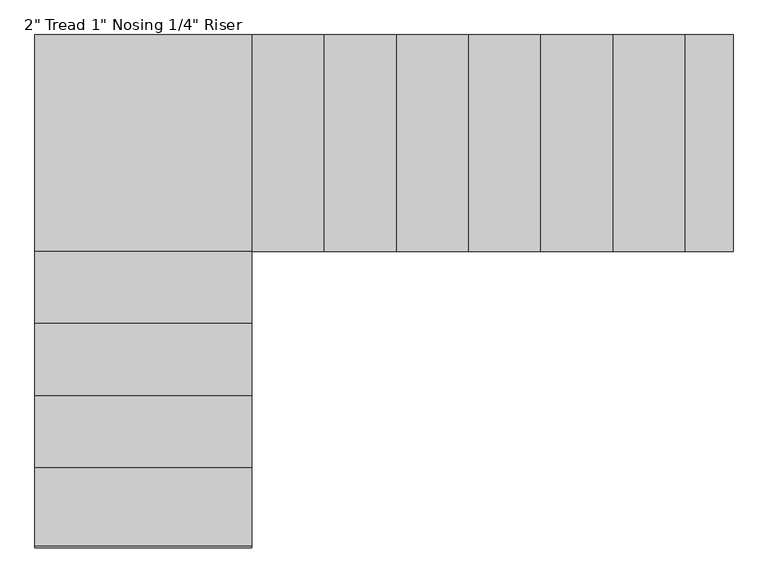
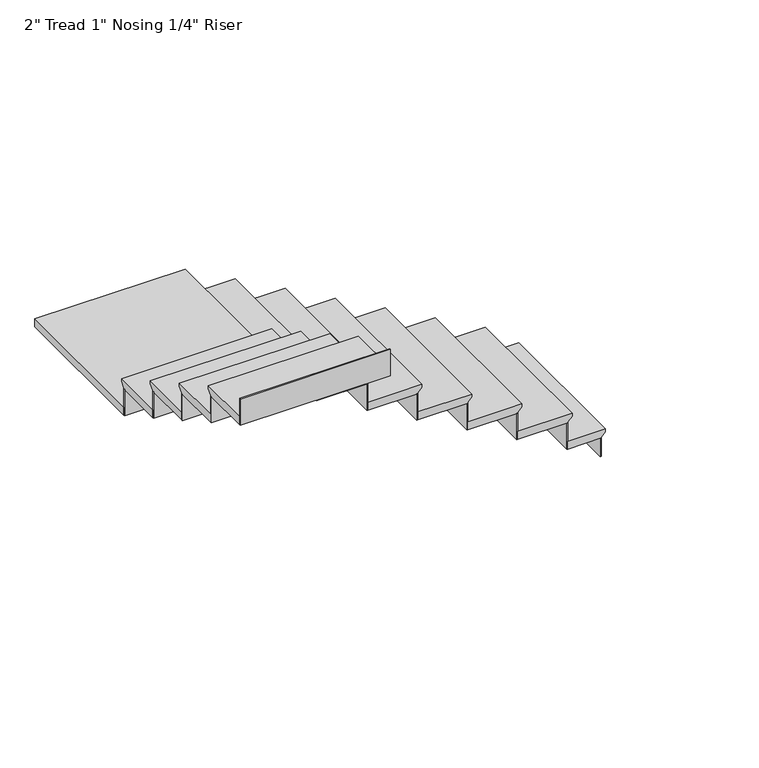
"""IFC4 building model written with IfcOpenShell, lengths in millimetres: stair flight geometry."""

from ifc_helpers import new_model, si_unit, origin, place, context, project, spatial, faceted_brep, source, transform, mapped, element, save


def stair_flight_1226b75b(model_context):
    return source(origin(), model_context, "Body", "Brep", [
        faceted_brep([(-442.4415084, 5282.3381995, 6398.6833333), (-442.4415084, 5282.3381995, 6417.7333333), (-442.4415084, 4368.3146777, 6417.7333333), (-442.4415084, 4368.3146777, 6398.6833333), (-467.8415084, 5282.3381995, 6373.2833333), (-467.8415084, 4368.3146777, 6373.2833333), (-671.0415084, 5282.3381995, 6417.7333333), (-671.0415084, 4368.3146777, 6417.7333333), (-467.8415084, 4368.3146777, 6366.9333333), (-671.0415084, 4368.3146777, 6366.9333333), (-671.0415084, 5282.3381995, 6366.9333333), (-467.8415084, 5282.3381995, 6366.9333333)], [[[0, 1, 2, 3]], [[4, 0, 3, 5]], [[2, 1, 6, 7]], [[8, 9, 10, 11]], [[2, 7, 9, 8, 5, 3]], [[8, 11, 4, 5]], [[6, 1, 0, 4, 11, 10]], [[7, 6, 10, 9]]]),
        faceted_brep([(-467.8415084, 5282.3381995, 6366.9333333), (-467.8415084, 5282.3381995, 6248.4), (-474.1915084, 5282.3381995, 6248.4), (-474.1915084, 5282.3381995, 6366.9333333), (-467.8415084, 4368.3146777, 6366.9333333), (-474.1915084, 4368.3146777, 6366.9333333), (-474.1915084, 4368.3146777, 6248.4), (-467.8415084, 4368.3146777, 6248.4)], [[[0, 1, 2, 3]], [[4, 5, 6, 7]], [[1, 0, 4, 7]], [[2, 1, 7, 6]], [[3, 2, 6, 5]], [[0, 3, 5, 4]]]),
        faceted_brep([(-671.0415084, 5282.3381995, 6536.2666667), (-671.0415084, 5282.3381995, 6366.9333333), (-677.3915084, 5282.3381995, 6366.9333333), (-677.3915084, 5282.3381995, 6536.2666667), (-671.0415084, 4368.3146777, 6536.2666667), (-677.3915084, 4368.3146777, 6536.2666667), (-677.3915084, 4368.3146777, 6366.9333333), (-671.0415084, 4368.3146777, 6366.9333333)], [[[0, 1, 2, 3]], [[4, 5, 6, 7]], [[1, 0, 4, 7]], [[2, 1, 7, 6]], [[3, 2, 6, 5]], [[0, 3, 5, 4]]]),
        faceted_brep([(-645.6415084, 4368.3146777, 6587.0666667), (-645.6415084, 5282.3381995, 6587.0666667), (-975.8415084, 5282.3381995, 6587.0666667), (-975.8415084, 4368.3146777, 6587.0666667), (-671.0415084, 4368.3146777, 6536.2666667), (-975.8415084, 4368.3146777, 6536.2666667), (-975.8415084, 5282.3381995, 6536.2666667), (-671.0415084, 5282.3381995, 6536.2666667), (-671.0415084, 4368.3146777, 6542.6166667), (-645.6415084, 4368.3146777, 6568.0166667), (-671.0415084, 5282.3381995, 6542.6166667), (-645.6415084, 5282.3381995, 6568.0166667)], [[[0, 1, 2, 3]], [[4, 5, 6, 7]], [[0, 3, 5, 4, 8, 9]], [[4, 7, 10, 8]], [[2, 1, 11, 10, 7, 6]], [[3, 2, 6, 5]], [[11, 1, 0, 9]], [[10, 11, 9, 8]]]),
        faceted_brep([(-975.8415084, 5282.3381995, 6705.6), (-975.8415084, 5282.3381995, 6536.2666667), (-982.1915084, 5282.3381995, 6536.2666667), (-982.1915084, 5282.3381995, 6705.6), (-975.8415084, 4368.3146777, 6705.6), (-982.1915084, 4368.3146777, 6705.6), (-982.1915084, 4368.3146777, 6536.2666667), (-975.8415084, 4368.3146777, 6536.2666667)], [[[0, 1, 2, 3]], [[4, 5, 6, 7]], [[1, 0, 4, 7]], [[2, 1, 7, 6]], [[3, 2, 6, 5]], [[0, 3, 5, 4]]]),
        faceted_brep([(-950.4415084, 4368.3146777, 6756.4), (-950.4415084, 5282.3381995, 6756.4), (-1280.6415084, 5282.3381995, 6756.4), (-1280.6415084, 4368.3146777, 6756.4), (-975.8415084, 4368.3146777, 6705.6), (-1280.6415084, 4368.3146777, 6705.6), (-1280.6415084, 5282.3381995, 6705.6), (-975.8415084, 5282.3381995, 6705.6), (-975.8415084, 4368.3146777, 6711.95), (-950.4415084, 4368.3146777, 6737.35), (-975.8415084, 5282.3381995, 6711.95), (-950.4415084, 5282.3381995, 6737.35)], [[[0, 1, 2, 3]], [[4, 5, 6, 7]], [[0, 3, 5, 4, 8, 9]], [[4, 7, 10, 8]], [[2, 1, 11, 10, 7, 6]], [[3, 2, 6, 5]], [[11, 1, 0, 9]], [[10, 11, 9, 8]]]),
        faceted_brep([(-1280.6415084, 5282.3381995, 6874.9333333), (-1280.6415084, 5282.3381995, 6705.6), (-1286.9915084, 5282.3381995, 6705.6), (-1286.9915084, 5282.3381995, 6874.9333333), (-1280.6415084, 4368.3146777, 6874.9333333), (-1286.9915084, 4368.3146777, 6874.9333333), (-1286.9915084, 4368.3146777, 6705.6), (-1280.6415084, 4368.3146777, 6705.6)], [[[0, 1, 2, 3]], [[4, 5, 6, 7]], [[1, 0, 4, 7]], [[2, 1, 7, 6]], [[3, 2, 6, 5]], [[0, 3, 5, 4]]]),
        faceted_brep([(-1255.2415084, 4368.3146777, 6925.7333333), (-1255.2415084, 5282.3381995, 6925.7333333), (-1585.4415084, 5282.3381995, 6925.7333333), (-1585.4415084, 4368.3146777, 6925.7333333), (-1280.6415084, 4368.3146777, 6874.9333333), (-1585.4415084, 4368.3146777, 6874.9333333), (-1585.4415084, 5282.3381995, 6874.9333333), (-1280.6415084, 5282.3381995, 6874.9333333), (-1280.6415084, 4368.3146777, 6881.2833333), (-1255.2415084, 4368.3146777, 6906.6833333), (-1280.6415084, 5282.3381995, 6881.2833333), (-1255.2415084, 5282.3381995, 6906.6833333)], [[[0, 1, 2, 3]], [[4, 5, 6, 7]], [[0, 3, 5, 4, 8, 9]], [[4, 7, 10, 8]], [[2, 1, 11, 10, 7, 6]], [[3, 2, 6, 5]], [[11, 1, 0, 9]], [[10, 11, 9, 8]]]),
        faceted_brep([(-1585.4415084, 5282.3381995, 7044.2666667), (-1585.4415084, 5282.3381995, 6874.9333333), (-1591.7915084, 5282.3381995, 6874.9333333), (-1591.7915084, 5282.3381995, 7044.2666667), (-1585.4415084, 4368.3146777, 7044.2666667), (-1591.7915084, 4368.3146777, 7044.2666667), (-1591.7915084, 4368.3146777, 6874.9333333), (-1585.4415084, 4368.3146777, 6874.9333333)], [[[0, 1, 2, 3]], [[4, 5, 6, 7]], [[1, 0, 4, 7]], [[2, 1, 7, 6]], [[3, 2, 6, 5]], [[0, 3, 5, 4]]]),
        faceted_brep([(-1560.0415084, 4368.3146777, 7095.0666667), (-1560.0415084, 5282.3381995, 7095.0666667), (-1890.2415084, 5282.3381995, 7095.0666667), (-1890.2415084, 4368.3146777, 7095.0666667), (-1585.4415084, 4368.3146777, 7044.2666667), (-1890.2415084, 4368.3146777, 7044.2666667), (-1890.2415084, 5282.3381995, 7044.2666667), (-1585.4415084, 5282.3381995, 7044.2666667), (-1585.4415084, 4368.3146777, 7050.6166667), (-1560.0415084, 4368.3146777, 7076.0166667), (-1585.4415084, 5282.3381995, 7050.6166667), (-1560.0415084, 5282.3381995, 7076.0166667)], [[[0, 1, 2, 3]], [[4, 5, 6, 7]], [[0, 3, 5, 4, 8, 9]], [[4, 7, 10, 8]], [[2, 1, 11, 10, 7, 6]], [[3, 2, 6, 5]], [[11, 1, 0, 9]], [[10, 11, 9, 8]]]),
        faceted_brep([(-1890.2415084, 5282.3381995, 7213.6), (-1890.2415084, 5282.3381995, 7044.2666667), (-1896.5915084, 5282.3381995, 7044.2666667), (-1896.5915084, 5282.3381995, 7213.6), (-1890.2415084, 4368.3146777, 7213.6), (-1896.5915084, 4368.3146777, 7213.6), (-1896.5915084, 4368.3146777, 7044.2666667), (-1890.2415084, 4368.3146777, 7044.2666667)], [[[0, 1, 2, 3]], [[4, 5, 6, 7]], [[1, 0, 4, 7]], [[2, 1, 7, 6]], [[3, 2, 6, 5]], [[0, 3, 5, 4]]]),
        faceted_brep([(-1864.8415084, 4368.3146777, 7264.4), (-1864.8415084, 5282.3381995, 7264.4), (-2195.0415084, 5282.3381995, 7264.4), (-2195.0415084, 4368.3146777, 7264.4), (-1890.2415084, 4368.3146777, 7213.6), (-2195.0415084, 4368.3146777, 7213.6), (-2195.0415084, 5282.3381995, 7213.6), (-1890.2415084, 5282.3381995, 7213.6), (-1890.2415084, 4368.3146777, 7219.95), (-1864.8415084, 4368.3146777, 7245.35), (-1890.2415084, 5282.3381995, 7219.95), (-1864.8415084, 5282.3381995, 7245.35)], [[[0, 1, 2, 3]], [[4, 5, 6, 7]], [[0, 3, 5, 4, 8, 9]], [[4, 7, 10, 8]], [[2, 1, 11, 10, 7, 6]], [[3, 2, 6, 5]], [[11, 1, 0, 9]], [[10, 11, 9, 8]]]),
        faceted_brep([(-2195.0415084, 5282.3381995, 7382.9333333), (-2195.0415084, 5282.3381995, 7213.6), (-2201.3915084, 5282.3381995, 7213.6), (-2201.3915084, 5282.3381995, 7382.9333333), (-2195.0415084, 4368.3146777, 7382.9333333), (-2201.3915084, 4368.3146777, 7382.9333333), (-2201.3915084, 4368.3146777, 7213.6), (-2195.0415084, 4368.3146777, 7213.6)], [[[0, 1, 2, 3]], [[4, 5, 6, 7]], [[1, 0, 4, 7]], [[2, 1, 7, 6]], [[3, 2, 6, 5]], [[0, 3, 5, 4]]]),
        faceted_brep([(-2169.6415084, 4368.3146777, 7433.7333333), (-2169.6415084, 5282.3381995, 7433.7333333), (-2499.8415084, 5282.3381995, 7433.7333333), (-2499.8415084, 4368.3146777, 7433.7333333), (-2195.0415084, 4368.3146777, 7382.9333333), (-2499.8415084, 4368.3146777, 7382.9333333), (-2499.8415084, 5282.3381995, 7382.9333333), (-2195.0415084, 5282.3381995, 7382.9333333), (-2195.0415084, 4368.3146777, 7389.2833333), (-2169.6415084, 4368.3146777, 7414.6833333), (-2195.0415084, 5282.3381995, 7389.2833333), (-2169.6415084, 5282.3381995, 7414.6833333)], [[[0, 1, 2, 3]], [[4, 5, 6, 7]], [[0, 3, 5, 4, 8, 9]], [[4, 7, 10, 8]], [[2, 1, 11, 10, 7, 6]], [[3, 2, 6, 5]], [[11, 1, 0, 9]], [[10, 11, 9, 8]]]),
        faceted_brep([(-2499.8415084, 5282.3381995, 7552.2666667), (-2499.8415084, 5282.3381995, 7382.9333333), (-2506.1915084, 5282.3381995, 7382.9333333), (-2506.1915084, 5282.3381995, 7552.2666667), (-2499.8415084, 4368.3146777, 7552.2666667), (-2506.1915084, 4368.3146777, 7552.2666667), (-2506.1915084, 4368.3146777, 7382.9333333), (-2499.8415084, 4368.3146777, 7382.9333333)], [[[0, 1, 2, 3]], [[4, 5, 6, 7]], [[1, 0, 4, 7]], [[2, 1, 7, 6]], [[3, 2, 6, 5]], [[0, 3, 5, 4]]]),
        faceted_brep([(-3388.8415084, 5282.3381995, 7603.0666667), (-3388.8415084, 4342.9146777, 7603.0666667), (-2474.4415084, 4342.9146777, 7603.0666667), (-2474.4415084, 5282.3381995, 7603.0666667), (-2474.4415084, 4368.3146777, 7552.2666667), (-2474.4415084, 4342.9146777, 7552.2666667), (-3388.8415084, 4342.9146777, 7552.2666667), (-3388.8415084, 5282.3381995, 7552.2666667), (-2499.8415084, 5282.3381995, 7552.2666667), (-2499.8415084, 4368.3146777, 7552.2666667), (-2474.4415084, 4368.3146777, 7584.0166667), (-2474.4415084, 5282.3381995, 7584.0166667), (-2499.8415084, 4368.3146777, 7558.6166667), (-2499.8415084, 5282.3381995, 7558.6166667)], [[[0, 1, 2, 3]], [[4, 5, 6, 7, 8, 9]], [[3, 2, 5, 4, 10, 11]], [[4, 9, 12, 10]], [[9, 8, 13, 12]], [[0, 3, 11, 13, 8, 7]], [[1, 0, 7, 6]], [[2, 1, 6, 5]], [[13, 11, 10, 12]]]),
        faceted_brep([(-3388.8415084, 4342.9146777, 7721.6), (-3388.8415084, 4342.9146777, 7552.2666667), (-3388.8415084, 4336.5646777, 7552.2666667), (-3388.8415084, 4336.5646777, 7721.6), (-2474.4415084, 4342.9146777, 7721.6), (-2474.4415084, 4336.5646777, 7721.6), (-2474.4415084, 4336.5646777, 7552.2666667), (-2474.4415084, 4342.9146777, 7552.2666667)], [[[0, 1, 2, 3]], [[4, 5, 6, 7]], [[1, 0, 4, 7]], [[2, 1, 7, 6]], [[3, 2, 6, 5]], [[0, 3, 5, 4]]]),
        faceted_brep([(-2474.4415084, 4368.3146777, 7772.4), (-3388.8415084, 4368.3146777, 7772.4), (-3388.8415084, 4037.7382512, 7772.4), (-2474.4415084, 4037.7382512, 7772.4), (-2474.4415084, 4342.9146777, 7721.6), (-2474.4415084, 4037.7382512, 7721.6), (-3388.8415084, 4037.7382512, 7721.6), (-3388.8415084, 4342.9146777, 7721.6), (-2474.4415084, 4342.9146777, 7727.95), (-2474.4415084, 4368.3146777, 7753.35), (-3388.8415084, 4342.9146777, 7727.95), (-3388.8415084, 4368.3146777, 7753.35)], [[[0, 1, 2, 3]], [[4, 5, 6, 7]], [[0, 3, 5, 4, 8, 9]], [[4, 7, 10, 8]], [[2, 1, 11, 10, 7, 6]], [[3, 2, 6, 5]], [[11, 1, 0, 9]], [[10, 11, 9, 8]]]),
        faceted_brep([(-3388.8415084, 4037.7382512, 7890.9333333), (-3388.8415084, 4037.7382512, 7721.6), (-3388.8415084, 4031.3882512, 7721.6), (-3388.8415084, 4031.3882512, 7890.9333333), (-2474.4415084, 4037.7382512, 7890.9333333), (-2474.4415084, 4031.3882512, 7890.9333333), (-2474.4415084, 4031.3882512, 7721.6), (-2474.4415084, 4037.7382512, 7721.6)], [[[0, 1, 2, 3]], [[4, 5, 6, 7]], [[1, 0, 4, 7]], [[2, 1, 7, 6]], [[3, 2, 6, 5]], [[0, 3, 5, 4]]]),
        faceted_brep([(-2474.4415084, 4063.1382512, 7941.7333333), (-3388.8415084, 4063.1382512, 7941.7333333), (-3388.8415084, 3732.938277, 7941.7333333), (-2474.4415084, 3732.938277, 7941.7333333), (-2474.4415084, 4037.7382512, 7890.9333333), (-2474.4415084, 3732.938277, 7890.9333333), (-3388.8415084, 3732.938277, 7890.9333333), (-3388.8415084, 4037.7382512, 7890.9333333), (-2474.4415084, 4037.7382512, 7897.2833333), (-2474.4415084, 4063.1382512, 7922.6833333), (-3388.8415084, 4037.7382512, 7897.2833333), (-3388.8415084, 4063.1382512, 7922.6833333)], [[[0, 1, 2, 3]], [[4, 5, 6, 7]], [[0, 3, 5, 4, 8, 9]], [[4, 7, 10, 8]], [[2, 1, 11, 10, 7, 6]], [[3, 2, 6, 5]], [[11, 1, 0, 9]], [[10, 11, 9, 8]]]),
        faceted_brep([(-3388.8415084, 3732.938277, 8060.2666667), (-3388.8415084, 3732.938277, 7890.9333333), (-3388.8415084, 3726.588277, 7890.9333333), (-3388.8415084, 3726.588277, 8060.2666667), (-2474.4415084, 3732.938277, 8060.2666667), (-2474.4415084, 3726.588277, 8060.2666667), (-2474.4415084, 3726.588277, 7890.9333333), (-2474.4415084, 3732.938277, 7890.9333333)], [[[0, 1, 2, 3]], [[4, 5, 6, 7]], [[1, 0, 4, 7]], [[2, 1, 7, 6]], [[3, 2, 6, 5]], [[0, 3, 5, 4]]]),
        faceted_brep([(-2474.4415084, 3758.338277, 8111.0666667), (-3388.8415084, 3758.338277, 8111.0666667), (-3388.8415084, 3428.1383028, 8111.0666667), (-2474.4415084, 3428.1383028, 8111.0666667), (-2474.4415084, 3732.938277, 8060.2666667), (-2474.4415084, 3428.1383028, 8060.2666667), (-3388.8415084, 3428.1383028, 8060.2666667), (-3388.8415084, 3732.938277, 8060.2666667), (-2474.4415084, 3732.938277, 8066.6166667), (-2474.4415084, 3758.338277, 8092.0166667), (-3388.8415084, 3732.938277, 8066.6166667), (-3388.8415084, 3758.338277, 8092.0166667)], [[[0, 1, 2, 3]], [[4, 5, 6, 7]], [[0, 3, 5, 4, 8, 9]], [[4, 7, 10, 8]], [[2, 1, 11, 10, 7, 6]], [[3, 2, 6, 5]], [[11, 1, 0, 9]], [[10, 11, 9, 8]]]),
        faceted_brep([(-3388.8415084, 3428.1383028, 8229.6), (-3388.8415084, 3428.1383028, 8060.2666667), (-3388.8415084, 3421.7883028, 8060.2666667), (-3388.8415084, 3421.7883028, 8229.6), (-2474.4415084, 3428.1383028, 8229.6), (-2474.4415084, 3421.7883028, 8229.6), (-2474.4415084, 3421.7883028, 8060.2666667), (-2474.4415084, 3428.1383028, 8060.2666667)], [[[0, 1, 2, 3]], [[4, 5, 6, 7]], [[1, 0, 4, 7]], [[2, 1, 7, 6]], [[3, 2, 6, 5]], [[0, 3, 5, 4]]]),
        faceted_brep([(-3388.8415084, 3123.3383287, 8398.9333333), (-3388.8415084, 3123.3383287, 8229.6), (-3388.8415084, 3116.9883287, 8229.6), (-3388.8415084, 3116.9883287, 8398.9333333), (-2474.4415084, 3123.3383287, 8398.9333333), (-2474.4415084, 3116.9883287, 8398.9333333), (-2474.4415084, 3116.9883287, 8229.6), (-2474.4415084, 3123.3383287, 8229.6)], [[[0, 1, 2, 3]], [[4, 5, 6, 7]], [[1, 0, 4, 7]], [[2, 1, 7, 6]], [[3, 2, 6, 5]], [[0, 3, 5, 4]]]),
        faceted_brep([(-2474.4415084, 3453.5383028, 8280.4), (-3388.8415084, 3453.5383028, 8280.4), (-3388.8415084, 3123.3383287, 8280.4), (-2474.4415084, 3123.3383287, 8280.4), (-2474.4415084, 3428.1383028, 8229.6), (-2474.4415084, 3123.3383287, 8229.6), (-3388.8415084, 3123.3383287, 8229.6), (-3388.8415084, 3428.1383028, 8229.6), (-2474.4415084, 3428.1383028, 8235.95), (-2474.4415084, 3453.5383028, 8261.35), (-3388.8415084, 3428.1383028, 8235.95), (-3388.8415084, 3453.5383028, 8261.35)], [[[0, 1, 2, 3]], [[4, 5, 6, 7]], [[0, 3, 5, 4, 8, 9]], [[4, 7, 10, 8]], [[2, 1, 11, 10, 7, 6]], [[3, 2, 6, 5]], [[11, 1, 0, 9]], [[10, 11, 9, 8]]]),
    ])


if __name__ == "__main__":
    model = new_model("IFC4")
    model_context = context("Model", 3, world=origin())
    ifc_project = project(units=[si_unit("LENGTHUNIT", "METRE", prefix="MILLI")], contexts=[model_context])
    site = spatial("IfcSite", under=ifc_project)
    building = spatial("IfcBuilding", under=site)
    placement = place(None, origin())
    stair_flight_shape = stair_flight_1226b75b(model_context)
    element("IfcStairFlight", 1, ObjectType="2\" Tread 1\" Nosing 1/4\" Riser", at=placement, inside=building, context=model_context, shape_type="MappedRepresentation", body=[
        mapped(stair_flight_shape, transform((0.0, 0.0, 0.0), x_axis=(1.0, 0.0, 0.0), y_axis=(0.0, 1.0, 0.0), z_axis=(0.0, 0.0, 1.0))),
    ])
    save(model, "model.ifc")
